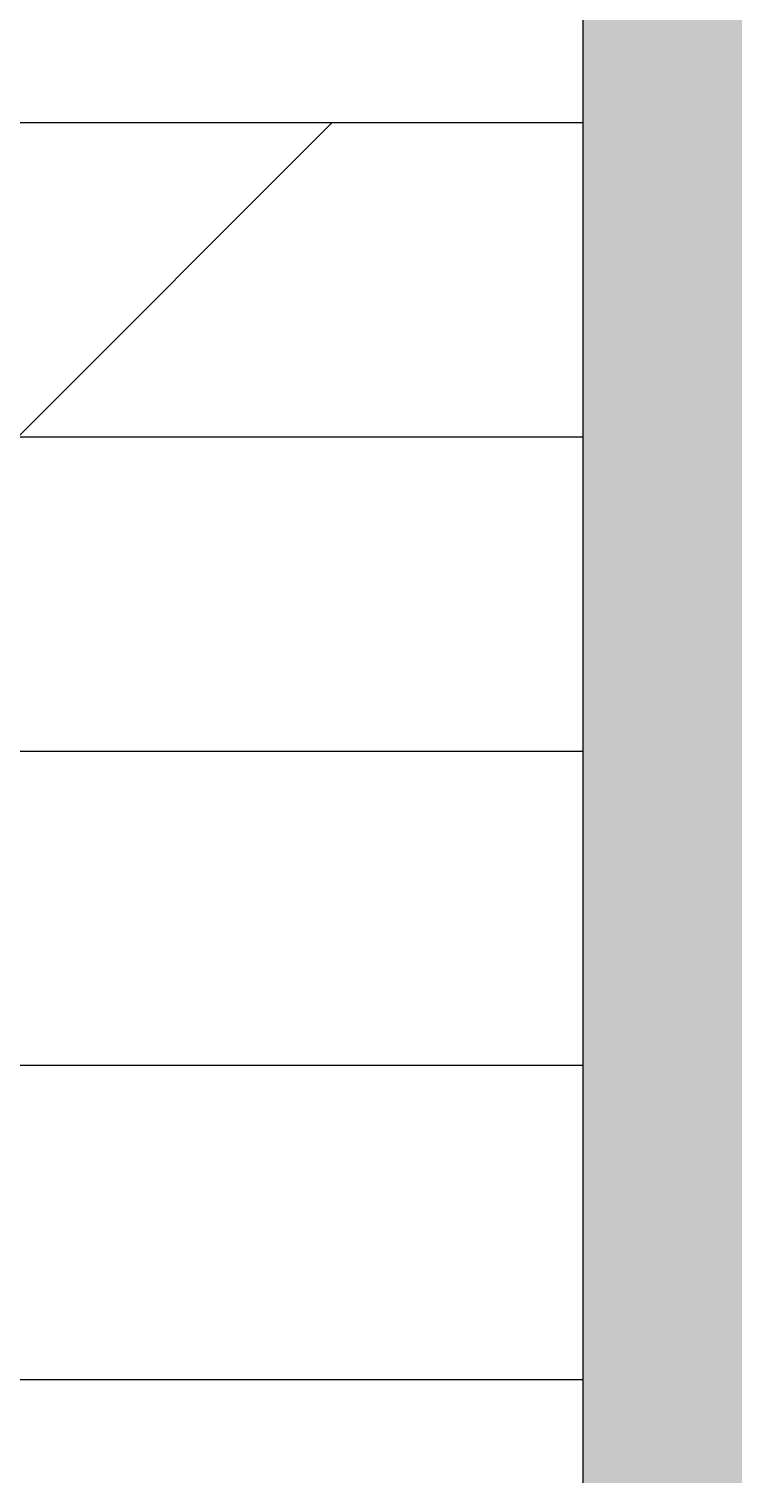
# Model space of a CAD drawing. Units: inches. Extents: x 84 to 1044, y -280 to 906.
# Tile 53 of 105: x 375 to 389, y 709 to 738. Entities that reach past the tile are written whole.
import ezdxf

# ---------------------------------------------------------------- set-up
doc = ezdxf.new("R2010")
doc.units = ezdxf.units.IN
doc.layers.add('A-ANNO-DIMS', color=2, linetype='Continuous', lineweight=18)
doc.layers.add('L-HRDS', color=32, linetype='Continuous', lineweight=18)
doc.layers.add('A-FLOR-PATT', color=251, linetype='Continuous', lineweight=9, true_color=0x705861)
doc.layers.add('L-PLNT-PATT', color=9, linetype='Continuous', lineweight=9, true_color=0xafd9aa)
doc.styles.get("Standard").update_dxf_attribs({"font": 'arial.ttf'})
doc.dimstyles.get("Standard").update_dxf_attribs({"dimtxt": 0.18, "dimasz": 0.18, "dimexe": 0.18, "dimexo": 0.0625, "dimgap": 0.09, "dimtad": 0, "dimtih": 1, "dimtoh": 1, "dimdec": 4, "dimzin": 0, "dimdsep": 46, "dimtxsty": 'Standard', "dimcen": 0.09, "dimadec": 0, "dimazin": 0, "dimtfac": 1, "dimtdec": 4, "dimtofl": 0, "dimtmove": 0, "dimatfit": 3, "dimfxl": 1, "dimtolj": 1, "dimtzin": 0, "dimarcsym": 0})

# ---------------------------------------------------------------- blocks, each defined once
blk = doc.blocks.new('*D62')
at = {"layer": 'A-ANNO-DIMS', "color": 0, "lineweight": -2, "transparency": 16777216}
for p, q in [((203.179, 709.183), (203.179, 905.9)), ((203.359, 905.72), (549.232, 905.72)), ((895.894, 905.72), (550.021, 905.72)), ((896.074, 400.183), (896.074, 905.9))]:
    blk.add_line(p, q, dxfattribs=at)
at = {"layer": 'A-ANNO-DIMS', "color": 0, "transparency": 16777216}
for points in [[(203.359, 905.75), (203.359, 905.69), (203.179, 905.72)], [(895.894, 905.75), (895.894, 905.69), (896.074, 905.72)]]:
    blk.add_solid(points, dxfattribs=at)
at = {"layer": 'Defpoints', "color": 0, "transparency": 16777216}
for p in [(896.074, 905.72), (203.179, 709.12), (896.074, 400.12)]:
    blk.add_point(p, dxfattribs=at)
at = {"layer": 'A-ANNO-DIMS', "color": 0, "transparency": 16777216, "insert": (549.627, 905.72), "char_height": 0.18, "attachment_point": 5}
blk.add_mtext('\\A1;692.9', dxfattribs=at)

msp = doc.modelspace()

# ---------------------------------------------------------------- hatches: boundary and pattern name
at = {"layer": 'A-FLOR-PATT', "transparency": 33554597}
h = msp.add_hatch(dxfattribs=at)
h.set_pattern_fill('DOLMIT', color=256)
h.paths.add_polyline_path([(896.074, 709.12), (833.074, 709.12), (833.074, 646.12), (833.074, 574.12), (833.074, 511.12), (896.074, 511.12)])
h.paths.add_polyline_path([(386.074, 769.12), (203.179, 769.12), (203.179, 709.12), (287.127, 709.12), (359.127, 709.12), (386.074, 709.12)])
at = {"layer": 'L-PLNT-PATT', "transparency": 33554597}
h = msp.add_hatch(color=256, dxfattribs=at)
h.dxf.hatch_style = 1
h.paths.add_polyline_path([(434.074, 769.12), (386.074, 769.12), (386.074, 709.12), (434.074, 709.12)])
h.paths.add_polyline_path([(896.074, 847.12), (434.074, 847.12), (434.074, 769.12), (434.074, 709.12), (470.074, 709.12), (506.074, 709.12), (572.074, 709.12), (608.074, 709.12), (698.074, 709.12), (770.074, 709.12), (833.074, 709.12), (896.074, 709.12)])
h.paths.add_polyline_path([(983.074, 847.12), (896.074, 847.12), (896.074, 709.12), (896.074, 547.12), (932.074, 547.12), (983.074, 547.12)])
h.paths.add_polyline_path([(983.074, 547.12), (932.074, 547.12), (932.074, 265.12), (983.074, 265.12)])
h.paths.add_polyline_path([(203.179, 646.12), (203.179, 709.12), (203.179, 745.12), (143.179, 745.12), (143.179, 271.12), (203.179, 271.12), (203.179, 274.12), (203.179, 310.12), (203.179, 574.12)])

# ---------------------------------------------------------------- linework, layer by layer
at = {"layer": 'L-HRDS'}
msp.add_line((386.074, 769.12), (386.074, 709.12), dxfattribs=at)

# ---------------------------------------------------------------- dimensions: what is measured, and where the dimension line sits
at = {"layer": 'A-ANNO-DIMS'}
dim = msp.add_linear_dim(base=(896.074, 905.72), p1=(203.179, 709.12), p2=(896.074, 400.12), dimstyle='Standard', override={"dimdec": 1, "dimlfac": 1, "dimrnd": 0, "dimzin": 0, "dimdsep": 46, "dimlunit": 2}, dxfattribs=at)
dim.commit()
dim.dimension.update_dxf_attribs({"geometry": '*D62', "text_midpoint": (549.627, 905.72)})

doc.saveas('drawing.dxf')
